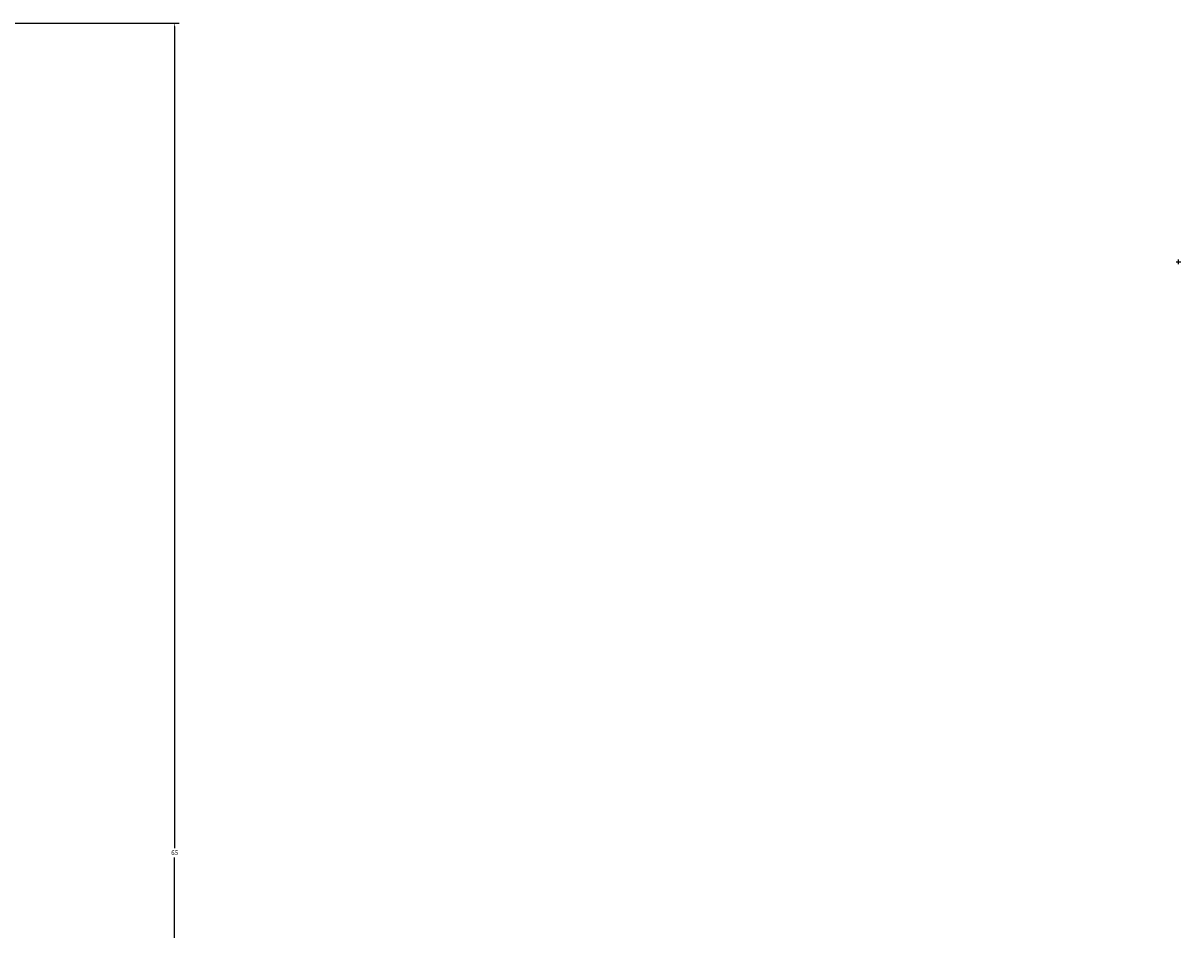
# Model space of a CAD drawing. Units: inches. Extents: x -13 to 107, y -48 to 102.
# Tile 13 of 13: x 62 to 107, y 43 to 78. Entities that reach past the tile are written whole.
import ezdxf

# ---------------------------------------------------------------- set-up
doc = ezdxf.new("R2010")
doc.units = ezdxf.units.IN
doc.header["$MEASUREMENT"] = 0
doc.layers.add('M-DIMS', color=2, linetype='Continuous', lineweight=18)
doc.styles.get("Standard").update_dxf_attribs({"font": 'arial.ttf'})
doc.dimstyles.get("Standard").update_dxf_attribs({"dimtxt": 0.18, "dimasz": 0.18, "dimexe": 0.18, "dimexo": 0.0625, "dimgap": 0.09, "dimtad": 0, "dimtih": 1, "dimtoh": 1, "dimdec": 4, "dimzin": 0, "dimdsep": 46, "dimtxsty": 'Standard', "dimcen": 0.09, "dimadec": 0, "dimazin": 0, "dimtfac": 1, "dimtdec": 4, "dimtofl": 0, "dimtmove": 0, "dimatfit": 3, "dimfxl": 1, "dimtolj": 1, "dimtzin": 0, "dimarcsym": 0})

# ---------------------------------------------------------------- blocks, each defined once
blk = doc.blocks.new('*D4')
at = {"layer": 'Defpoints', "color": 0, "transparency": 16777216}
for p in [(27.547, 78.408), (67.679, 78.408), (27.547, 13.408)]:
    blk.add_point(p, dxfattribs=at)
at = {"layer": 'M-DIMS', "color": 0, "lineweight": -2, "transparency": 16777216}
for p, q in [((27.609, 78.408), (67.859, 78.408)), ((67.679, 78.228), (67.679, 46.09)), ((67.679, 13.588), (67.679, 45.726)), ((27.609, 13.408), (67.859, 13.408))]:
    blk.add_line(p, q, dxfattribs=at)
at = {"layer": 'M-DIMS', "color": 0, "transparency": 16777216}
for points in [[(67.649, 78.228), (67.709, 78.228), (67.679, 78.408)], [(67.649, 13.588), (67.709, 13.588), (67.679, 13.408)]]:
    blk.add_solid(points, dxfattribs=at)
at = {"layer": 'M-DIMS', "color": 0, "transparency": 16777216, "insert": (67.679, 45.908), "char_height": 0.18, "attachment_point": 5}
blk.add_mtext('\\A1;65', dxfattribs=at)
blk = doc.blocks.new('*D14')
at = {"layer": 'Defpoints', "color": 0, "transparency": 16777216}
for p in [(106.998, 69.054), (43.126, 65.005)]:
    blk.add_point(p, dxfattribs=at)
at = {"layer": 'M-DIMS', "color": 0, "lineweight": -2, "transparency": 16777216}
for p, q in [((106.908, 69.054), (107.088, 69.054)), ((106.998, 68.964), (106.998, 69.144)), ((4.803, 62.576), (42.947, 64.994))]:
    blk.add_line(p, q, dxfattribs=at)
at = {"layer": 'M-DIMS', "color": 0, "transparency": 16777216}
blk.add_solid([(42.945, 65.024), (42.949, 64.964), (43.126, 65.005)], dxfattribs=at)
at = {"layer": 'M-DIMS', "color": 0, "transparency": 16777216, "insert": (4.304, 62.576), "char_height": 0.18, "attachment_point": 5}
blk.add_mtext('\\A1;2X R64', dxfattribs=at)

msp = doc.modelspace()

# ---------------------------------------------------------------- dimensions: what is measured, and where the dimension line sits
at = {"layer": 'M-DIMS'}
dim = msp.add_linear_dim(base=(67.679, 78.408), p1=(27.547, 13.408), p2=(27.547, 78.408), angle=90, dimstyle='Standard', override={"dimdec": 0, "dimlfac": 1, "dimrnd": 0, "dimzin": 0, "dimdsep": 46, "dimlunit": 2}, dxfattribs=at)
dim.commit()
dim.dimension.update_dxf_attribs({"geometry": '*D4', "text_midpoint": (67.679, 45.908)})
dim = msp.add_radius_dim(center=(106.998, 69.054), mpoint=(43.126, 65.005), text='2X <>', dimstyle='Standard', override={"dimdec": 0, "dimlfac": 1, "dimrnd": 0, "dimzin": 0, "dimdsep": 46, "dimlunit": 2}, dxfattribs=at)
dim.commit()
dim.dimension.update_dxf_attribs({"geometry": '*D14', "text_midpoint": (4.803, 62.576), "dimtype": 164})

doc.saveas('drawing.dxf')
